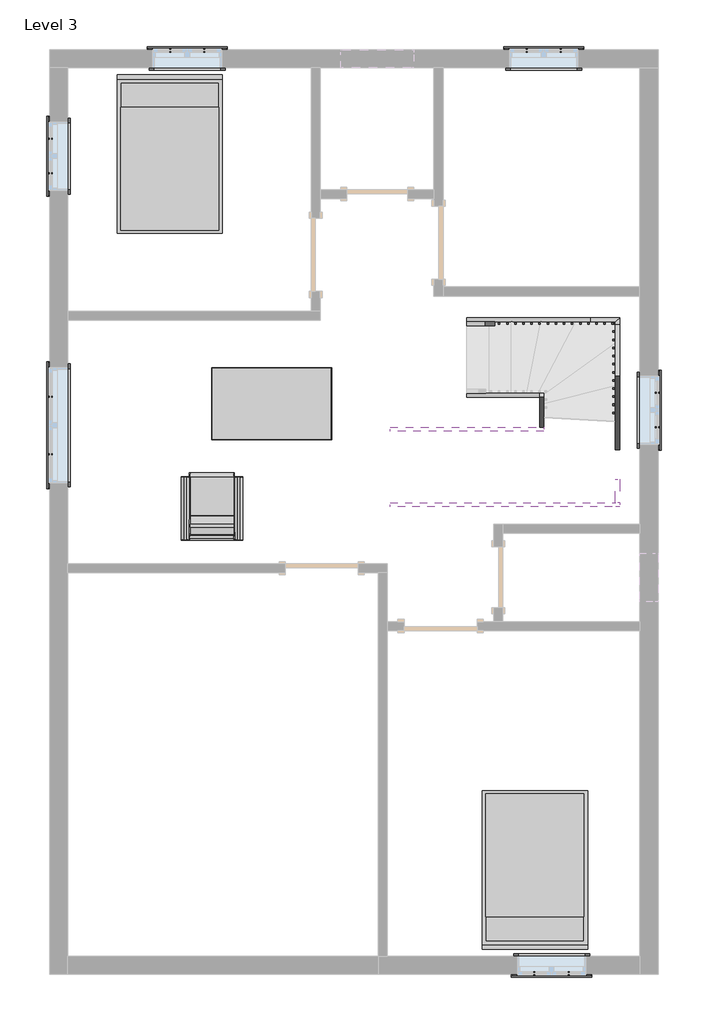
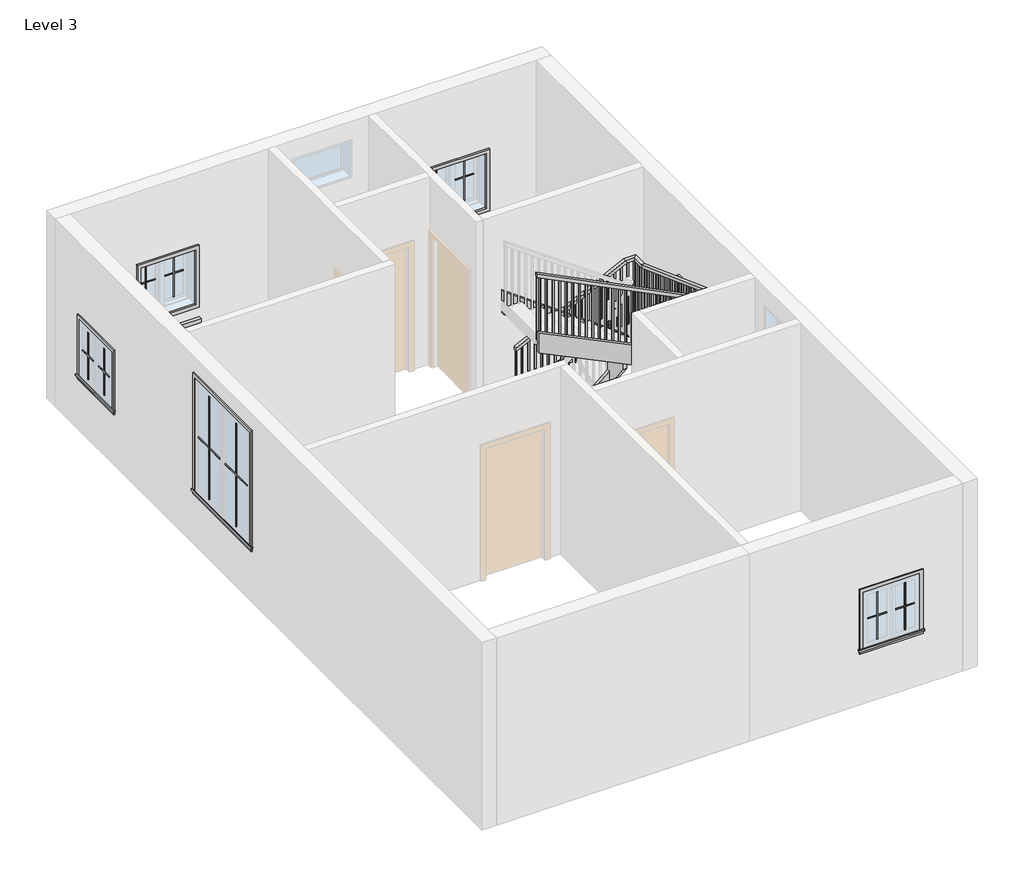
# One storey, part 2 of 2: 24 proxies, 9 members, 4 furniture elements, 1 railing.
"""IFC4 building model written with IfcOpenShell, lengths in millimetres."""

from ifc_helpers import new_model, si_unit, frame, origin, place, context, project, spatial, polyline, outline, extrude, faceted_brep, transform, mapped, element, save
from components import muntin_pattern_2x2_muntin_pattern_2x2_b3fe6957, muntin_pattern_2x2_muntin_pattern_2x2_3e0ecaf2, muntin_pattern_2x2_muntin_pattern_2x2_bff912c5, muntin_pattern_2x2_muntin_pattern_2x2_c2194282, trim_window_exterior_flat_with_sill_41619996, trim_window_exterior_flat_with_sill_e04b3088, trim_window_interior_flat_picture_frame_51c85655, trim_window_interior_flat_picture_frame_2a7685fe, furniture_f28dd14e, furniture_402a1f5e, bed_17739_bed_17739_15c61121, dining_table_14755_dining_table_14755_d89cb775

model = new_model("IFC4")

# Units and contexts
model_context = context("Model", 3, world=origin())
ifc_project = project(units=[si_unit("LENGTHUNIT", "METRE", prefix="MILLI")], contexts=[model_context])

# Site, building, storey
site = spatial("IfcSite", under=ifc_project)
building = spatial("IfcBuilding", under=site)
storey = spatial("IfcBuildingStorey", under=building, Name="Level 3", Elevation=3200.4)

# Proxies
placement = place(None, origin())
muntin_pattern_2x2_muntin_pattern_2x2_shape = muntin_pattern_2x2_muntin_pattern_2x2_b3fe6957(model_context)
element("IfcBuildingElementProxy", 1, Name="Muntin Pattern_2x2 : Muntin Pattern_2x2", ObjectType="Muntin Pattern_2x2 : Muntin Pattern_2x2", at=placement, inside=storey, context=model_context, shape_type="MappedRepresentation", body=[
    mapped(muntin_pattern_2x2_muntin_pattern_2x2_shape, transform((-3555.5290084, 6319.8685985, 4184.65), x_axis=(1.0, 0.0, 0.0), y_axis=(0.0, 1.0, 0.0), z_axis=(0.0, 0.0, 1.0))),
])
element("IfcBuildingElementProxy", 2, Name="Muntin Pattern_2x2 : Muntin Pattern_2x2", ObjectType="Muntin Pattern_2x2 : Muntin Pattern_2x2", at=placement, inside=storey, context=model_context, shape_type="MappedRepresentation", body=[
    mapped(muntin_pattern_2x2_muntin_pattern_2x2_shape, transform((1435.5709916, -5243.4814015, 4184.65), x_axis=(-1.0, 0.0, 0.0), y_axis=(0.0, -1.0, 0.0), z_axis=(0.0, 0.0, 1.0))),
])
element("IfcBuildingElementProxy", 3, Name="Muntin Pattern_2x2 : Muntin Pattern_2x2", ObjectType="Muntin Pattern_2x2 : Muntin Pattern_2x2", at=placement, inside=storey, context=model_context, shape_type="MappedRepresentation", body=[
    mapped(muntin_pattern_2x2_muntin_pattern_2x2_shape, transform((2545.2334916, 2028.8560985, 4184.65), x_axis=(0.0, -1.0, 0.0), y_axis=(1.0, 0.0, 0.0), z_axis=(0.0, 0.0, 1.0))),
])
element("IfcBuildingElementProxy", 4, Name="Muntin Pattern_2x2 : Muntin Pattern_2x2", ObjectType="Muntin Pattern_2x2 : Muntin Pattern_2x2", at=placement, inside=storey, context=model_context, shape_type="MappedRepresentation", body=[
    mapped(muntin_pattern_2x2_muntin_pattern_2x2_shape, transform((908.5209916, 6319.8685985, 4184.65), x_axis=(1.0, 0.0, 0.0), y_axis=(0.0, 1.0, 0.0), z_axis=(0.0, 0.0, 1.0))),
])
element("IfcBuildingElementProxy", 5, Name="Muntin Pattern_2x2 : Muntin Pattern_2x2", ObjectType="Muntin Pattern_2x2 : Muntin Pattern_2x2", at=placement, inside=storey, context=model_context, shape_type="MappedRepresentation", body=[
    mapped(muntin_pattern_2x2_muntin_pattern_2x2_shape, transform((-5055.7165084, 4781.5810985, 4184.65), x_axis=(0.0, 1.0, 0.0), y_axis=(-1.0, 0.0, 0.0), z_axis=(0.0, 0.0, 1.0))),
])
muntin_pattern_2x2_muntin_pattern_2x2_2_shape = muntin_pattern_2x2_muntin_pattern_2x2_3e0ecaf2(model_context)
element("IfcBuildingElementProxy", 6, Name="Muntin Pattern_2x2 : Muntin Pattern_2x2", ObjectType="Muntin Pattern_2x2 : Muntin Pattern_2x2", at=placement, inside=storey, context=model_context, shape_type="MappedRepresentation", body=[
    mapped(muntin_pattern_2x2_muntin_pattern_2x2_2_shape, transform((-3126.9040084, 6319.8685985, 4184.65), x_axis=(-1.0, 0.0, 0.0), y_axis=(0.0, -1.0, 0.0), z_axis=(0.0, 0.0, 1.0))),
])
element("IfcBuildingElementProxy", 7, Name="Muntin Pattern_2x2 : Muntin Pattern_2x2", ObjectType="Muntin Pattern_2x2 : Muntin Pattern_2x2", at=placement, inside=storey, context=model_context, shape_type="MappedRepresentation", body=[
    mapped(muntin_pattern_2x2_muntin_pattern_2x2_2_shape, transform((1006.9459916, -5243.4814015, 4184.65), x_axis=(1.0, 0.0, 0.0), y_axis=(0.0, 1.0, 0.0), z_axis=(0.0, 0.0, 1.0))),
])
element("IfcBuildingElementProxy", 8, Name="Muntin Pattern_2x2 : Muntin Pattern_2x2", ObjectType="Muntin Pattern_2x2 : Muntin Pattern_2x2", at=placement, inside=storey, context=model_context, shape_type="MappedRepresentation", body=[
    mapped(muntin_pattern_2x2_muntin_pattern_2x2_2_shape, transform((2545.2334916, 1600.2310985, 4184.65), x_axis=(0.0, 1.0, 0.0), y_axis=(-1.0, 0.0, 0.0), z_axis=(0.0, 0.0, 1.0))),
])
element("IfcBuildingElementProxy", 9, Name="Muntin Pattern_2x2 : Muntin Pattern_2x2", ObjectType="Muntin Pattern_2x2 : Muntin Pattern_2x2", at=placement, inside=storey, context=model_context, shape_type="MappedRepresentation", body=[
    mapped(muntin_pattern_2x2_muntin_pattern_2x2_2_shape, transform((1337.1459916, 6319.8685985, 4184.65), x_axis=(-1.0, 0.0, 0.0), y_axis=(0.0, -1.0, 0.0), z_axis=(0.0, 0.0, 1.0))),
])
element("IfcBuildingElementProxy", 10, Name="Muntin Pattern_2x2 : Muntin Pattern_2x2", ObjectType="Muntin Pattern_2x2 : Muntin Pattern_2x2", at=placement, inside=storey, context=model_context, shape_type="MappedRepresentation", body=[
    mapped(muntin_pattern_2x2_muntin_pattern_2x2_2_shape, transform((-5055.7165084, 5210.2060985, 4184.65), x_axis=(0.0, -1.0, 0.0), y_axis=(1.0, 0.0, 0.0), z_axis=(0.0, 0.0, 1.0))),
])
muntin_pattern_2x2_muntin_pattern_2x2_3_shape = muntin_pattern_2x2_muntin_pattern_2x2_bff912c5(model_context)
element("IfcBuildingElementProxy", 11, Name="Muntin Pattern_2x2 : Muntin Pattern_2x2", ObjectType="Muntin Pattern_2x2 : Muntin Pattern_2x2", at=placement, inside=storey, context=model_context, shape_type="MappedRepresentation", body=[
    mapped(muntin_pattern_2x2_muntin_pattern_2x2_3_shape, transform((-5055.7165084, 1263.6810985, 4184.65), x_axis=(0.0, 1.0, 0.0), y_axis=(-1.0, 0.0, 0.0), z_axis=(0.0, 0.0, 1.0))),
])
muntin_pattern_2x2_muntin_pattern_2x2_4_shape = muntin_pattern_2x2_muntin_pattern_2x2_c2194282(model_context)
element("IfcBuildingElementProxy", 12, Name="Muntin Pattern_2x2 : Muntin Pattern_2x2", ObjectType="Muntin Pattern_2x2 : Muntin Pattern_2x2", at=placement, inside=storey, context=model_context, shape_type="MappedRepresentation", body=[
    mapped(muntin_pattern_2x2_muntin_pattern_2x2_4_shape, transform((-5055.7165084, 1984.4060985, 4184.65), x_axis=(0.0, -1.0, 0.0), y_axis=(1.0, 0.0, 0.0), z_axis=(0.0, 0.0, 1.0))),
])
trim_window_exterior_flat_with_sill_shape = trim_window_exterior_flat_with_sill_41619996(model_context)
element("IfcBuildingElementProxy", 13, Name="Trim-Window-Exterior-Flat : with Sill", ObjectType="Trim-Window-Exterior-Flat : with Sill", at=placement, inside=storey, context=model_context, shape_type="MappedRepresentation", body=[
    mapped(trim_window_exterior_flat_with_sill_shape, transform((-3341.2165084, 6329.3935985, 5029.2), x_axis=(-1.0, 0.0, 0.0), y_axis=(0.0, 0.0, 1.0), z_axis=(0.0, 1.0, 0.0))),
])
element("IfcBuildingElementProxy", 14, Name="Trim-Window-Exterior-Flat : with Sill", ObjectType="Trim-Window-Exterior-Flat : with Sill", at=placement, inside=storey, context=model_context, shape_type="MappedRepresentation", body=[
    mapped(trim_window_exterior_flat_with_sill_shape, transform((1221.2584916, -5253.0064015, 5029.2), x_axis=(1.0, 0.0, 0.0), y_axis=(0.0, 0.0, 1.0), z_axis=(0.0, -1.0, 0.0))),
])
element("IfcBuildingElementProxy", 15, Name="Trim-Window-Exterior-Flat : with Sill", ObjectType="Trim-Window-Exterior-Flat : with Sill", at=placement, inside=storey, context=model_context, shape_type="MappedRepresentation", body=[
    mapped(trim_window_exterior_flat_with_sill_shape, transform((2554.7584916, 1814.5435985, 5029.2), x_axis=(0.0, 1.0, 0.0), y_axis=(0.0, 0.0, 1.0), z_axis=(1.0, 0.0, 0.0))),
])
element("IfcBuildingElementProxy", 16, Name="Trim-Window-Exterior-Flat : with Sill", ObjectType="Trim-Window-Exterior-Flat : with Sill", at=placement, inside=storey, context=model_context, shape_type="MappedRepresentation", body=[
    mapped(trim_window_exterior_flat_with_sill_shape, transform((1122.8334916, 6329.3935985, 5029.2), x_axis=(-1.0, 0.0, 0.0), y_axis=(0.0, 0.0, 1.0), z_axis=(0.0, 1.0, 0.0))),
])
element("IfcBuildingElementProxy", 17, Name="Trim-Window-Exterior-Flat : with Sill", ObjectType="Trim-Window-Exterior-Flat : with Sill", at=placement, inside=storey, context=model_context, shape_type="MappedRepresentation", body=[
    mapped(trim_window_exterior_flat_with_sill_shape, transform((-5065.2415084, 4995.8935985, 5029.2), x_axis=(0.0, -1.0, 0.0), y_axis=(0.0, 0.0, 1.0), z_axis=(-1.0, 0.0, 0.0))),
])
trim_window_exterior_flat_with_sill_2_shape = trim_window_exterior_flat_with_sill_e04b3088(model_context)
element("IfcBuildingElementProxy", 18, Name="Trim-Window-Exterior-Flat : with Sill", ObjectType="Trim-Window-Exterior-Flat : with Sill", at=placement, inside=storey, context=model_context, shape_type="MappedRepresentation", body=[
    mapped(trim_window_exterior_flat_with_sill_2_shape, transform((-5065.2415084, 1624.0435985, 5943.6), x_axis=(0.0, -1.0, 0.0), y_axis=(0.0, 0.0, 1.0), z_axis=(-1.0, 0.0, 0.0))),
])
trim_window_interior_flat_picture_frame_shape = trim_window_interior_flat_picture_frame_51c85655(model_context)
element("IfcBuildingElementProxy", 19, Name="Trim-Window-Interior-Flat : Picture Frame", ObjectType="Trim-Window-Interior-Flat : Picture Frame", at=placement, inside=storey, context=model_context, shape_type="MappedRepresentation", body=[
    mapped(trim_window_interior_flat_picture_frame_shape, transform((-3341.2165084, 6100.7935985, 5029.2), x_axis=(1.0, 0.0, 0.0), y_axis=(0.0, 0.0, 1.0), z_axis=(0.0, -1.0, 0.0))),
])
element("IfcBuildingElementProxy", 20, Name="Trim-Window-Interior-Flat : Picture Frame", ObjectType="Trim-Window-Interior-Flat : Picture Frame", at=placement, inside=storey, context=model_context, shape_type="MappedRepresentation", body=[
    mapped(trim_window_interior_flat_picture_frame_shape, transform((1221.2584916, -5024.4064015, 5029.2), x_axis=(-1.0, 0.0, 0.0), y_axis=(0.0, 0.0, 1.0), z_axis=(0.0, 1.0, 0.0))),
])
element("IfcBuildingElementProxy", 21, Name="Trim-Window-Interior-Flat : Picture Frame", ObjectType="Trim-Window-Interior-Flat : Picture Frame", at=placement, inside=storey, context=model_context, shape_type="MappedRepresentation", body=[
    mapped(trim_window_interior_flat_picture_frame_shape, transform((2326.1584916, 1814.5435985, 5029.2), x_axis=(0.0, -1.0, 0.0), y_axis=(0.0, 0.0, 1.0), z_axis=(-1.0, 0.0, 0.0))),
])
element("IfcBuildingElementProxy", 22, Name="Trim-Window-Interior-Flat : Picture Frame", ObjectType="Trim-Window-Interior-Flat : Picture Frame", at=placement, inside=storey, context=model_context, shape_type="MappedRepresentation", body=[
    mapped(trim_window_interior_flat_picture_frame_shape, transform((1122.8334916, 6100.7935985, 5029.2), x_axis=(1.0, 0.0, 0.0), y_axis=(0.0, 0.0, 1.0), z_axis=(0.0, -1.0, 0.0))),
])
element("IfcBuildingElementProxy", 23, Name="Trim-Window-Interior-Flat : Picture Frame", ObjectType="Trim-Window-Interior-Flat : Picture Frame", at=placement, inside=storey, context=model_context, shape_type="MappedRepresentation", body=[
    mapped(trim_window_interior_flat_picture_frame_shape, transform((-4836.6415084, 4995.8935985, 5029.2), x_axis=(0.0, 1.0, 0.0), y_axis=(0.0, 0.0, 1.0), z_axis=(1.0, 0.0, 0.0))),
])
trim_window_interior_flat_picture_frame_2_shape = trim_window_interior_flat_picture_frame_2a7685fe(model_context)
element("IfcBuildingElementProxy", 24, Name="Trim-Window-Interior-Flat : Picture Frame", ObjectType="Trim-Window-Interior-Flat : Picture Frame", at=placement, inside=storey, context=model_context, shape_type="MappedRepresentation", body=[
    mapped(trim_window_interior_flat_picture_frame_2_shape, transform((-4836.6415084, 1624.0435985, 5943.6), x_axis=(0.0, 1.0, 0.0), y_axis=(0.0, 0.0, 1.0), z_axis=(1.0, 0.0, 0.0))),
])

# Furniture
furniture_shape = furniture_f28dd14e(model_context)
furniture_2_shape = furniture_402a1f5e(model_context)
element("IfcFurniture", 25, at=placement, inside=storey, context=model_context, shape_type="MappedRepresentation", body=[
    mapped(furniture_shape, transform((-3032.3877006, 981.9349825, 3200.4), x_axis=(-1.0, 0.0, 0.0), y_axis=(0.0, -1.0, 0.0), z_axis=(0.0, 0.0, 1.0))),
    mapped(furniture_2_shape, transform((-3032.3877006, 981.9349825, 3200.4), x_axis=(-1.0, 0.0, 0.0), y_axis=(0.0, -1.0, 0.0), z_axis=(0.0, 0.0, 1.0))),
])
bed_17739_bed_17739_shape = bed_17739_bed_17739_15c61121(model_context)
element("IfcFurniture", 26, ObjectType="Bed_17739 : Bed_17739", at=placement, inside=storey, context=model_context, shape_type="MappedRepresentation", body=[
    mapped(bed_17739_bed_17739_shape, transform((-3560.2915084, 4995.8935985, 3200.4), x_axis=(1.0, 0.0, 0.0), y_axis=(0.0, 1.0, 0.0), z_axis=(0.0, 0.0, 1.0))),
])
element("IfcFurniture", 27, ObjectType="Bed_17739 : Bed_17739", at=placement, inside=storey, context=model_context, shape_type="MappedRepresentation", body=[
    mapped(bed_17739_bed_17739_shape, transform((1011.7084916, -3919.5064015, 3200.4), x_axis=(-1.0, 0.0, 0.0), y_axis=(0.0, -1.0, 0.0), z_axis=(0.0, 0.0, 1.0))),
])
dining_table_14755_dining_table_14755_shape = dining_table_14755_dining_table_14755_d89cb775(model_context)
element("IfcFurniture", 28, ObjectType="Dining_table_14755 : Dining_table_14755", at=placement, inside=storey, context=model_context, shape_type="MappedRepresentation", body=[
    mapped(dining_table_14755_dining_table_14755_shape, transform((-3032.3877006, 1444.8879061, 3200.4), x_axis=(1.0, 0.0, 0.0), y_axis=(0.0, 1.0, 0.0), z_axis=(0.0, 0.0, 1.0))),
])

# Members
element("IfcMember", 29, ObjectType="Stringer - 2\" Width", at=placement, inside=storey, context=model_context, shape_type="SweptSolid", body=[
    extrude(outline(polyline([(3439.8504763, 158.6923968), (3200.4, 158.6923968), (3200.4, 366.2169505), (3826.6639814, 1705.9967367), (4163.1193197, 1705.9967367), (3439.8504763, 158.6923968)])), frame((0.0, 2922.8476133, 0.0), z_axis=(0.0, 1.0, 0.0), x_axis=(0.0, 0.0, 1.0)), (0.0, 0.0, 1.0), 50.8),
])
element("IfcMember", 30, ObjectType="Stringer - 2\" Width", at=placement, inside=storey, context=model_context, shape_type="SweptSolid", body=[
    extrude(outline(polyline([(1705.9967367, 2922.8476133), (1705.9967367, 2973.6476133), (2072.9441983, 2973.6476133), (2022.1441983, 2922.8476133), (1705.9967367, 2922.8476133)])), frame((0.0, 0.0, 3826.6639814), z_axis=(0.0, 0.0, 1.0), x_axis=(1.0, 0.0, 0.0)), (0.0, 0.0, 1.0), 336.4553383),
])
element("IfcMember", 31, ObjectType="Stringer - 2\" Width", at=placement, inside=storey, context=model_context, shape_type="SweptSolid", body=[
    extrude(outline(polyline([(2022.1441983, 2922.8476133), (2072.9441983, 2973.6476133), (2072.9441983, 2883.4348143), (2022.1441983, 2883.4348143), (2022.1441983, 2922.8476133)])), frame((0.0, 0.0, 3826.6639814), z_axis=(0.0, 0.0, 1.0), x_axis=(1.0, 0.0, 0.0)), (0.0, 0.0, 1.0), 336.4553383),
])
element("IfcMember", 32, ObjectType="Stringer - 2\" Width", at=placement, inside=storey, context=model_context, shape_type="SweptSolid", body=[
    extrude(outline(polyline([(2883.4348143, 4163.1193197), (2883.4348143, 3826.6639814), (947.0260734, 4536.0990218), (947.0260734, 4872.5543601), (2883.4348143, 4163.1193197)])), frame((2022.1441983, 0.0, 0.0), z_axis=(1.0, 0.0, 0.0), x_axis=(0.0, 1.0, 0.0)), (0.0, 0.0, 1.0), 50.8),
])
element("IfcMember", 33, ObjectType="Stringer - 2\" Width", at=placement, inside=storey, context=model_context, shape_type="SweptSolid", body=[
    extrude(outline(polyline([(2022.1441983, 947.0260734), (2072.9441983, 947.0260734), (2072.9441983, 652.4935985), (2022.1441983, 652.4935985), (2022.1441983, 947.0260734)])), frame((0.0, 0.0, 4541.7754285), z_axis=(0.0, 0.0, 1.0), x_axis=(1.0, 0.0, 0.0)), (0.0, 0.0, 1.0), 324.6119022),
])
element("IfcMember", 34, ObjectType="Stringer - 2\" Width", at=placement, inside=storey, context=model_context, shape_type="SweptSolid", body=[
    extrude(outline(polyline([(3374.8551137, 158.6923968), (3200.4, 158.6923968), (3200.4, 426.0767146), (3734.5870321, 1072.5901835), (4129.9706215, 1072.5901835), (3374.8551137, 158.6923968)])), frame((0.0, 1973.2935985, 0.0), z_axis=(0.0, 1.0, 0.0), x_axis=(0.0, 0.0, 1.0)), (0.0, 0.0, 1.0), 50.8),
])
element("IfcMember", 35, ObjectType="Stringer - 2\" Width", at=placement, inside=storey, context=model_context, shape_type="SweptSolid", body=[
    extrude(outline(polyline([(2024.0935985, 4333.296008), (2024.0935985, 3830.5724164), (1602.0476133, 4384.1407029), (1602.0476133, 4886.8642945), (2024.0935985, 4333.296008)])), frame((1072.5901835, 0.0, 0.0), z_axis=(1.0, 0.0, 0.0), x_axis=(0.0, 1.0, 0.0)), (0.0, 0.0, 1.0), 50.8),
])
element("IfcMember", 36, ObjectType="Stringer - 2\" Width", at=placement, inside=storey, context=model_context, shape_type="SweptSolid", body=[
    extrude(outline(polyline([(4562.5113348, 1123.3901835), (4939.4379401, 1123.3901835), (6337.5009734, -798.3242294), (5960.5743681, -798.3242294), (4562.5113348, 1123.3901835)])), frame((0.0, 1551.2476133, 0.0), z_axis=(0.0, 1.0, 0.0), x_axis=(0.0, 0.0, 1.0)), (0.0, 0.0, 1.0), 50.8),
])
element("IfcMember", 37, ObjectType="Stringer - 2\" Width", at=placement, inside=storey, context=model_context, shape_type="SweptSolid", body=[
    extrude(outline(polyline([(4561.5873308, 2072.9441983), (4841.6397747, 2072.9441983), (6240.3971818, -798.3242294), (5915.7852796, -798.3242294), (4561.5873308, 1981.4757528), (4561.5873308, 2072.9441983)])), frame((0.0, 601.6935985, 0.0), z_axis=(0.0, 1.0, 0.0), x_axis=(0.0, 0.0, 1.0)), (0.0, 0.0, 1.0), 50.8),
])

# Railing
element("IfcRailing", 38, ObjectType="Handrail - Rectangular", at=placement, inside=storey, context=model_context, shape_type="SolidModel", body=[
    faceted_brep([(158.6923968, 2922.8476133, 4284.1333333), (158.6923968, 2922.8476133, 4227.4325724), (158.6923968, 2872.0476133, 4227.4325724), (158.6923968, 2872.0476133, 4284.1333333), (1841.0143863, 2922.8476133, 5118.2084972), (1852.9161672, 2922.8476133, 5067.4084972), (1852.9161672, 2872.0476133, 5067.4084972), (1841.0143863, 2872.0476133, 5118.2084972), (2022.1441983, 2922.8476133, 5118.2084972), (2022.1441983, 2922.8476133, 5067.4084972), (1971.3441983, 2872.0476133, 5067.4084972), (1971.3441983, 2872.0476133, 5118.2084972), (2022.1441983, 2686.7050655, 5118.2084972), (2022.1441983, 2677.692274, 5067.4084972), (1971.3441983, 2677.692274, 5067.4084972), (1971.3441983, 2686.7050655, 5118.2084972), (2022.1441983, 796.951655, 5810.5505936), (2022.1441983, 787.9388635, 5759.7505936), (1971.3441983, 787.9388635, 5759.7505936), (1971.3441983, 796.951655, 5810.5505936), (2022.1441983, 652.4935985, 5810.5505936), (2022.1441983, 652.4935985, 5759.7505936), (1971.3441983, 703.2935985, 5759.7505936), (1971.3441983, 703.2935985, 5810.5505936), (1909.402346, 652.4935985, 5810.5505936), (1897.4228813, 652.4935985, 5759.7505936), (1897.4228813, 703.2935985, 5759.7505936), (1909.402346, 703.2935985, 5810.5505936), (-798.3242294, 652.4935985, 7162.8), (-798.3242294, 703.2935985, 7162.8), (-798.3242294, 703.2935985, 7106.0174077), (-798.3242294, 652.4935985, 7106.0174077)], [[[0, 1, 2, 3]], [[1, 0, 4, 5]], [[2, 1, 5, 6]], [[3, 2, 6, 7]], [[0, 3, 7, 4]], [[5, 4, 8, 9]], [[6, 5, 9, 10]], [[7, 6, 10, 11]], [[4, 7, 11, 8]], [[9, 8, 12, 13]], [[10, 9, 13, 14]], [[11, 10, 14, 15]], [[8, 11, 15, 12]], [[13, 12, 16, 17]], [[14, 13, 17, 18]], [[15, 14, 18, 19]], [[12, 15, 19, 16]], [[17, 16, 20, 21]], [[18, 17, 21, 22]], [[19, 18, 22, 23]], [[16, 19, 23, 20]], [[21, 20, 24, 25]], [[22, 21, 25, 26]], [[23, 22, 26, 27]], [[20, 23, 27, 24]], [[28, 29, 30, 31]], [[25, 24, 28, 31]], [[26, 25, 31, 30]], [[27, 26, 30, 29]], [[24, 27, 29, 28]]]),
    extrude(outline(polyline([(7084.8709318, -755.9808017), (6079.0666667, -755.9808017), (6079.0666667, -736.9308017), (7075.3572862, -736.9308017), (7084.8709318, -755.9808017)])), frame((0.0, 668.3685985, 0.0), z_axis=(0.0, 1.0, 0.0), x_axis=(0.0, 0.0, 1.0)), (0.0, 0.0, 1.0), 19.05),
    extrude(outline(polyline([(7034.1314883, -654.3808017), (6079.0666667, -654.3808017), (6079.0666667, -635.3308017), (7024.6178426, -635.3308017), (7034.1314883, -654.3808017)])), frame((0.0, 668.3685985, 0.0), z_axis=(0.0, 1.0, 0.0), x_axis=(0.0, 0.0, 1.0)), (0.0, 0.0, 1.0), 19.05),
    extrude(outline(polyline([(6983.3920447, -552.7808017), (6079.0666667, -552.7808017), (6079.0666667, -533.7308017), (6973.8783991, -533.7308017), (6983.3920447, -552.7808017)])), frame((0.0, 668.3685985, 0.0), z_axis=(0.0, 1.0, 0.0), x_axis=(0.0, 0.0, 1.0)), (0.0, 0.0, 1.0), 19.05),
    extrude(outline(polyline([(6932.6526012, -451.1808017), (5909.7333333, -451.1808017), (5909.7333333, -432.1308017), (6923.1389555, -432.1308017), (6932.6526012, -451.1808017)])), frame((0.0, 668.3685985, 0.0), z_axis=(0.0, 1.0, 0.0), x_axis=(0.0, 0.0, 1.0)), (0.0, 0.0, 1.0), 19.05),
    extrude(outline(polyline([(6881.9131577, -349.5808017), (5909.7333333, -349.5808017), (5909.7333333, -330.5308017), (6872.399512, -330.5308017), (6881.9131577, -349.5808017)])), frame((0.0, 668.3685985, 0.0), z_axis=(0.0, 1.0, 0.0), x_axis=(0.0, 0.0, 1.0)), (0.0, 0.0, 1.0), 19.05),
    extrude(outline(polyline([(6831.1737141, -247.9808017), (5740.4, -247.9808017), (5740.4, -228.9308017), (6821.6600685, -228.9308017), (6831.1737141, -247.9808017)])), frame((0.0, 668.3685985, 0.0), z_axis=(0.0, 1.0, 0.0), x_axis=(0.0, 0.0, 1.0)), (0.0, 0.0, 1.0), 19.05),
    extrude(outline(polyline([(6780.4342706, -146.3808017), (5740.4, -146.3808017), (5740.4, -127.3308017), (6770.9206249, -127.3308017), (6780.4342706, -146.3808017)])), frame((0.0, 668.3685985, 0.0), z_axis=(0.0, 1.0, 0.0), x_axis=(0.0, 0.0, 1.0)), (0.0, 0.0, 1.0), 19.05),
    extrude(outline(polyline([(6729.694827, -44.7808017), (5740.4, -44.7808017), (5740.4, -25.7308017), (6720.1811814, -25.7308017), (6729.694827, -44.7808017)])), frame((0.0, 668.3685985, 0.0), z_axis=(0.0, 1.0, 0.0), x_axis=(0.0, 0.0, 1.0)), (0.0, 0.0, 1.0), 19.05),
    extrude(outline(polyline([(6678.9553835, 56.8191983), (5571.0666667, 56.8191983), (5571.0666667, 75.8691983), (6669.4417378, 75.8691983), (6678.9553835, 56.8191983)])), frame((0.0, 668.3685985, 0.0), z_axis=(0.0, 1.0, 0.0), x_axis=(0.0, 0.0, 1.0)), (0.0, 0.0, 1.0), 19.05),
    extrude(outline(polyline([(6628.21594, 158.4191983), (5571.0666667, 158.4191983), (5571.0666667, 177.4691983), (6618.7022943, 177.4691983), (6628.21594, 158.4191983)])), frame((0.0, 668.3685985, 0.0), z_axis=(0.0, 1.0, 0.0), x_axis=(0.0, 0.0, 1.0)), (0.0, 0.0, 1.0), 19.05),
    extrude(outline(polyline([(6577.4764964, 260.0191983), (5571.0666667, 260.0191983), (5571.0666667, 279.0691983), (6567.9628508, 279.0691983), (6577.4764964, 260.0191983)])), frame((0.0, 668.3685985, 0.0), z_axis=(0.0, 1.0, 0.0), x_axis=(0.0, 0.0, 1.0)), (0.0, 0.0, 1.0), 19.05),
    extrude(outline(polyline([(6526.7370529, 361.6191983), (5401.7333333, 361.6191983), (5401.7333333, 380.6691983), (6517.2234072, 380.6691983), (6526.7370529, 361.6191983)])), frame((0.0, 668.3685985, 0.0), z_axis=(0.0, 1.0, 0.0), x_axis=(0.0, 0.0, 1.0)), (0.0, 0.0, 1.0), 19.05),
    extrude(outline(polyline([(6475.9976093, 463.2191983), (5401.7333333, 463.2191983), (5401.7333333, 482.2691983), (6466.4839637, 482.2691983), (6475.9976093, 463.2191983)])), frame((0.0, 668.3685985, 0.0), z_axis=(0.0, 1.0, 0.0), x_axis=(0.0, 0.0, 1.0)), (0.0, 0.0, 1.0), 19.05),
    extrude(outline(polyline([(6425.2581658, 564.8191983), (5401.7333333, 564.8191983), (5401.7333333, 583.8691983), (6415.7445201, 583.8691983), (6425.2581658, 564.8191983)])), frame((0.0, 668.3685985, 0.0), z_axis=(0.0, 1.0, 0.0), x_axis=(0.0, 0.0, 1.0)), (0.0, 0.0, 1.0), 19.05),
    extrude(outline(polyline([(6374.5187223, 666.4191983), (5232.4, 666.4191983), (5232.4, 685.4691983), (6365.0050766, 685.4691983), (6374.5187223, 666.4191983)])), frame((0.0, 668.3685985, 0.0), z_axis=(0.0, 1.0, 0.0), x_axis=(0.0, 0.0, 1.0)), (0.0, 0.0, 1.0), 19.05),
    extrude(outline(polyline([(6323.7792787, 768.0191983), (5232.4, 768.0191983), (5232.4, 787.0691983), (6314.265633, 787.0691983), (6323.7792787, 768.0191983)])), frame((0.0, 668.3685985, 0.0), z_axis=(0.0, 1.0, 0.0), x_axis=(0.0, 0.0, 1.0)), (0.0, 0.0, 1.0), 19.05),
    extrude(outline(polyline([(6273.0398352, 869.6191983), (5232.4, 869.6191983), (5232.4, 888.6691983), (6263.5261895, 888.6691983), (6273.0398352, 869.6191983)])), frame((0.0, 668.3685985, 0.0), z_axis=(0.0, 1.0, 0.0), x_axis=(0.0, 0.0, 1.0)), (0.0, 0.0, 1.0), 19.05),
    extrude(outline(polyline([(6222.3003916, 971.2191983), (5232.4, 971.2191983), (5232.4, 990.2691983), (6212.786746, 990.2691983), (6222.3003916, 971.2191983)])), frame((0.0, 668.3685985, 0.0), z_axis=(0.0, 1.0, 0.0), x_axis=(0.0, 0.0, 1.0)), (0.0, 0.0, 1.0), 19.05),
    extrude(outline(polyline([(6171.5609481, 1072.8191983), (5063.0666667, 1072.8191983), (5063.0666667, 1091.8691983), (6162.0473024, 1091.8691983), (6171.5609481, 1072.8191983)])), frame((0.0, 668.3685985, 0.0), z_axis=(0.0, 1.0, 0.0), x_axis=(0.0, 0.0, 1.0)), (0.0, 0.0, 1.0), 19.05),
    extrude(outline(polyline([(6120.8215046, 1174.4191983), (5063.0666667, 1174.4191983), (5063.0666667, 1193.4691983), (6111.3078589, 1193.4691983), (6120.8215046, 1174.4191983)])), frame((0.0, 668.3685985, 0.0), z_axis=(0.0, 1.0, 0.0), x_axis=(0.0, 0.0, 1.0)), (0.0, 0.0, 1.0), 19.05),
    extrude(outline(polyline([(6070.082061, 1276.0191983), (5063.0666667, 1276.0191983), (5063.0666667, 1295.0691983), (6060.5684153, 1295.0691983), (6070.082061, 1276.0191983)])), frame((0.0, 668.3685985, 0.0), z_axis=(0.0, 1.0, 0.0), x_axis=(0.0, 0.0, 1.0)), (0.0, 0.0, 1.0), 19.05),
    extrude(outline(polyline([(6019.3426175, 1377.6191983), (4893.7333333, 1377.6191983), (4893.7333333, 1396.6691983), (6009.8289718, 1396.6691983), (6019.3426175, 1377.6191983)])), frame((0.0, 668.3685985, 0.0), z_axis=(0.0, 1.0, 0.0), x_axis=(0.0, 0.0, 1.0)), (0.0, 0.0, 1.0), 19.05),
    extrude(outline(polyline([(5968.6031739, 1479.2191983), (4893.7333333, 1479.2191983), (4893.7333333, 1498.2691983), (5959.0895283, 1498.2691983), (5968.6031739, 1479.2191983)])), frame((0.0, 668.3685985, 0.0), z_axis=(0.0, 1.0, 0.0), x_axis=(0.0, 0.0, 1.0)), (0.0, 0.0, 1.0), 19.05),
    extrude(outline(polyline([(5917.8637304, 1580.8191983), (4893.7333333, 1580.8191983), (4893.7333333, 1599.8691983), (5908.3500847, 1599.8691983), (5917.8637304, 1580.8191983)])), frame((0.0, 668.3685985, 0.0), z_axis=(0.0, 1.0, 0.0), x_axis=(0.0, 0.0, 1.0)), (0.0, 0.0, 1.0), 19.05),
    extrude(outline(polyline([(5867.1242869, 1682.4191983), (4893.7333333, 1682.4191983), (4893.7333333, 1701.4691983), (5857.6106412, 1701.4691983), (5867.1242869, 1682.4191983)])), frame((0.0, 668.3685985, 0.0), z_axis=(0.0, 1.0, 0.0), x_axis=(0.0, 0.0, 1.0)), (0.0, 0.0, 1.0), 19.05),
    extrude(outline(polyline([(5816.3848433, 1784.0191983), (4893.7333333, 1784.0191983), (4893.7333333, 1803.0691983), (5806.8711976, 1803.0691983), (5816.3848433, 1784.0191983)])), frame((0.0, 668.3685985, 0.0), z_axis=(0.0, 1.0, 0.0), x_axis=(0.0, 0.0, 1.0)), (0.0, 0.0, 1.0), 19.05),
    extrude(outline(polyline([(5765.6453998, 1885.6191983), (4724.4, 1885.6191983), (4724.4, 1904.6691983), (5756.1317541, 1904.6691983), (5765.6453998, 1885.6191983)])), frame((0.0, 668.3685985, 0.0), z_axis=(0.0, 1.0, 0.0), x_axis=(0.0, 0.0, 1.0)), (0.0, 0.0, 1.0), 19.05),
    extrude(outline(polyline([(2006.2691983, 773.3726133), (2006.2691983, 754.3226133), (1987.2191983, 754.3226133), (1987.2191983, 773.3726133), (2006.2691983, 773.3726133)])), frame((0.0, 0.0, 4724.4), z_axis=(0.0, 0.0, 1.0), x_axis=(1.0, 0.0, 0.0)), (0.0, 0.0, 1.0), 1035.3505936),
    extrude(outline(polyline([(874.9726133, 5727.8643546), (874.9726133, 4724.4), (855.9226133, 4724.4), (855.9226133, 5734.843634), (874.9726133, 5727.8643546)])), frame((1987.2191983, 0.0, 0.0), z_axis=(1.0, 0.0, 0.0), x_axis=(0.0, 1.0, 0.0)), (0.0, 0.0, 1.0), 19.05),
    extrude(outline(polyline([(976.5726133, 5690.6415315), (976.5726133, 4724.4), (957.5226133, 4724.4), (957.5226133, 5697.6208108), (976.5726133, 5690.6415315)])), frame((1987.2191983, 0.0, 0.0), z_axis=(1.0, 0.0, 0.0), x_axis=(0.0, 1.0, 0.0)), (0.0, 0.0, 1.0), 19.05),
    extrude(outline(polyline([(1078.1726133, 5653.4187083), (1078.1726133, 4724.4), (1059.1226133, 4724.4), (1059.1226133, 5660.3979877), (1078.1726133, 5653.4187083)])), frame((1987.2191983, 0.0, 0.0), z_axis=(1.0, 0.0, 0.0), x_axis=(0.0, 1.0, 0.0)), (0.0, 0.0, 1.0), 19.05),
    extrude(outline(polyline([(1179.7726133, 5616.1958852), (1179.7726133, 4724.4), (1160.7226133, 4724.4), (1160.7226133, 5623.1751645), (1179.7726133, 5616.1958852)])), frame((1987.2191983, 0.0, 0.0), z_axis=(1.0, 0.0, 0.0), x_axis=(0.0, 1.0, 0.0)), (0.0, 0.0, 1.0), 19.05),
    extrude(outline(polyline([(1281.3726133, 5578.973062), (1281.3726133, 4724.4), (1262.3226133, 4724.4), (1262.3226133, 5585.9523414), (1281.3726133, 5578.973062)])), frame((1987.2191983, 0.0, 0.0), z_axis=(1.0, 0.0, 0.0), x_axis=(0.0, 1.0, 0.0)), (0.0, 0.0, 1.0), 19.05),
    extrude(outline(polyline([(1382.9726133, 5541.7502389), (1382.9726133, 4555.0666667), (1363.9226133, 4555.0666667), (1363.9226133, 5548.7295182), (1382.9726133, 5541.7502389)])), frame((1987.2191983, 0.0, 0.0), z_axis=(1.0, 0.0, 0.0), x_axis=(0.0, 1.0, 0.0)), (0.0, 0.0, 1.0), 19.05),
    extrude(outline(polyline([(1484.5726133, 5504.5274157), (1484.5726133, 4555.0666667), (1465.5226133, 4555.0666667), (1465.5226133, 5511.5066951), (1484.5726133, 5504.5274157)])), frame((1987.2191983, 0.0, 0.0), z_axis=(1.0, 0.0, 0.0), x_axis=(0.0, 1.0, 0.0)), (0.0, 0.0, 1.0), 19.05),
    extrude(outline(polyline([(1586.1726133, 5467.3045926), (1586.1726133, 4555.0666667), (1567.1226133, 4555.0666667), (1567.1226133, 5474.2838719), (1586.1726133, 5467.3045926)])), frame((1987.2191983, 0.0, 0.0), z_axis=(1.0, 0.0, 0.0), x_axis=(0.0, 1.0, 0.0)), (0.0, 0.0, 1.0), 19.05),
    extrude(outline(polyline([(1687.7726133, 5430.0817694), (1687.7726133, 4555.0666667), (1668.7226133, 4555.0666667), (1668.7226133, 5437.0610488), (1687.7726133, 5430.0817694)])), frame((1987.2191983, 0.0, 0.0), z_axis=(1.0, 0.0, 0.0), x_axis=(0.0, 1.0, 0.0)), (0.0, 0.0, 1.0), 19.05),
    extrude(outline(polyline([(1789.3726133, 5392.8589463), (1789.3726133, 4385.7333333), (1770.3226133, 4385.7333333), (1770.3226133, 5399.8382256), (1789.3726133, 5392.8589463)])), frame((1987.2191983, 0.0, 0.0), z_axis=(1.0, 0.0, 0.0), x_axis=(0.0, 1.0, 0.0)), (0.0, 0.0, 1.0), 19.05),
    extrude(outline(polyline([(1890.9726133, 5355.6361231), (1890.9726133, 4385.7333333), (1871.9226133, 4385.7333333), (1871.9226133, 5362.6154025), (1890.9726133, 5355.6361231)])), frame((1987.2191983, 0.0, 0.0), z_axis=(1.0, 0.0, 0.0), x_axis=(0.0, 1.0, 0.0)), (0.0, 0.0, 1.0), 19.05),
    extrude(outline(polyline([(1992.5726133, 5318.4133), (1992.5726133, 4385.7333333), (1973.5226133, 4385.7333333), (1973.5226133, 5325.3925793), (1992.5726133, 5318.4133)])), frame((1987.2191983, 0.0, 0.0), z_axis=(1.0, 0.0, 0.0), x_axis=(0.0, 1.0, 0.0)), (0.0, 0.0, 1.0), 19.05),
    extrude(outline(polyline([(2094.1726133, 5281.1904769), (2094.1726133, 4385.7333333), (2075.1226133, 4385.7333333), (2075.1226133, 5288.1697562), (2094.1726133, 5281.1904769)])), frame((1987.2191983, 0.0, 0.0), z_axis=(1.0, 0.0, 0.0), x_axis=(0.0, 1.0, 0.0)), (0.0, 0.0, 1.0), 19.05),
    extrude(outline(polyline([(2195.7726133, 5243.9676537), (2195.7726133, 4216.4), (2176.7226133, 4216.4), (2176.7226133, 5250.946933), (2195.7726133, 5243.9676537)])), frame((1987.2191983, 0.0, 0.0), z_axis=(1.0, 0.0, 0.0), x_axis=(0.0, 1.0, 0.0)), (0.0, 0.0, 1.0), 19.05),
    extrude(outline(polyline([(2297.3726133, 5206.7448306), (2297.3726133, 4216.4), (2278.3226133, 4216.4), (2278.3226133, 5213.7241099), (2297.3726133, 5206.7448306)])), frame((1987.2191983, 0.0, 0.0), z_axis=(1.0, 0.0, 0.0), x_axis=(0.0, 1.0, 0.0)), (0.0, 0.0, 1.0), 19.05),
    extrude(outline(polyline([(2398.9726133, 5169.5220074), (2398.9726133, 4216.4), (2379.9226133, 4216.4), (2379.9226133, 5176.5012867), (2398.9726133, 5169.5220074)])), frame((1987.2191983, 0.0, 0.0), z_axis=(1.0, 0.0, 0.0), x_axis=(0.0, 1.0, 0.0)), (0.0, 0.0, 1.0), 19.05),
    extrude(outline(polyline([(2500.5726133, 5132.2991843), (2500.5726133, 4216.4), (2481.5226133, 4216.4), (2481.5226133, 5139.2784636), (2500.5726133, 5132.2991843)])), frame((1987.2191983, 0.0, 0.0), z_axis=(1.0, 0.0, 0.0), x_axis=(0.0, 1.0, 0.0)), (0.0, 0.0, 1.0), 19.05),
    extrude(outline(polyline([(2602.1726133, 5095.0763611), (2602.1726133, 4216.4), (2583.1226133, 4216.4), (2583.1226133, 5102.0556405), (2602.1726133, 5095.0763611)])), frame((1987.2191983, 0.0, 0.0), z_axis=(1.0, 0.0, 0.0), x_axis=(0.0, 1.0, 0.0)), (0.0, 0.0, 1.0), 19.05),
    extrude(outline(polyline([(2006.2691983, 2703.7726133), (2006.2691983, 2684.7226133), (1987.2191983, 2684.7226133), (1987.2191983, 2703.7726133), (2006.2691983, 2703.7726133)])), frame((0.0, 0.0, 4047.0666667), z_axis=(0.0, 0.0, 1.0), x_axis=(1.0, 0.0, 0.0)), (0.0, 0.0, 1.0), 1020.3418305),
    extrude(outline(polyline([(2006.2691983, 2805.3726133), (2006.2691983, 2786.3226133), (1987.2191983, 2786.3226133), (1987.2191983, 2805.3726133), (2006.2691983, 2805.3726133)])), frame((0.0, 0.0, 4047.0666667), z_axis=(0.0, 0.0, 1.0), x_axis=(1.0, 0.0, 0.0)), (0.0, 0.0, 1.0), 1020.3418305),
    extrude(outline(polyline([(1977.9673968, 2906.9726133), (1997.0173968, 2906.9726133), (1997.0173968, 2887.9226133), (1977.9673968, 2887.9226133), (1977.9673968, 2906.9726133)])), frame((0.0, 0.0, 4047.0666667), z_axis=(0.0, 0.0, 1.0), x_axis=(1.0, 0.0, 0.0)), (0.0, 0.0, 1.0), 1020.3418305),
    extrude(outline(polyline([(1876.3673968, 2906.9726133), (1895.4173968, 2906.9726133), (1895.4173968, 2887.9226133), (1876.3673968, 2887.9226133), (1876.3673968, 2906.9726133)])), frame((0.0, 0.0, 4047.0666667), z_axis=(0.0, 0.0, 1.0), x_axis=(1.0, 0.0, 0.0)), (0.0, 0.0, 1.0), 1020.3418305),
    extrude(outline(polyline([(5028.6632695, 1774.7673968), (4047.0666667, 1774.7673968), (4047.0666667, 1793.8173968), (5038.1080321, 1793.8173968), (5028.6632695, 1774.7673968)])), frame((0.0, 2887.9226133, 0.0), z_axis=(0.0, 1.0, 0.0), x_axis=(0.0, 0.0, 1.0)), (0.0, 0.0, 1.0), 19.05),
    extrude(outline(polyline([(4978.2912021, 1673.1673968), (4047.0666667, 1673.1673968), (4047.0666667, 1692.2173968), (4987.7359647, 1692.2173968), (4978.2912021, 1673.1673968)])), frame((0.0, 2887.9226133, 0.0), z_axis=(0.0, 1.0, 0.0), x_axis=(0.0, 0.0, 1.0)), (0.0, 0.0, 1.0), 19.05),
    extrude(outline(polyline([(4927.9191347, 1571.5673968), (4047.0666667, 1571.5673968), (4047.0666667, 1590.6173968), (4937.3638973, 1590.6173968), (4927.9191347, 1571.5673968)])), frame((0.0, 2887.9226133, 0.0), z_axis=(0.0, 1.0, 0.0), x_axis=(0.0, 0.0, 1.0)), (0.0, 0.0, 1.0), 19.05),
    extrude(outline(polyline([(4877.5470673, 1469.9673968), (3877.7333333, 1469.9673968), (3877.7333333, 1489.0173968), (4886.9918299, 1489.0173968), (4877.5470673, 1469.9673968)])), frame((0.0, 2887.9226133, 0.0), z_axis=(0.0, 1.0, 0.0), x_axis=(0.0, 0.0, 1.0)), (0.0, 0.0, 1.0), 19.05),
    extrude(outline(polyline([(4827.1749999, 1368.3673968), (3877.7333333, 1368.3673968), (3877.7333333, 1387.4173968), (4836.6197625, 1387.4173968), (4827.1749999, 1368.3673968)])), frame((0.0, 2887.9226133, 0.0), z_axis=(0.0, 1.0, 0.0), x_axis=(0.0, 0.0, 1.0)), (0.0, 0.0, 1.0), 19.05),
    extrude(outline(polyline([(4776.8029325, 1266.7673968), (3877.7333333, 1266.7673968), (3877.7333333, 1285.8173968), (4786.2476951, 1285.8173968), (4776.8029325, 1266.7673968)])), frame((0.0, 2887.9226133, 0.0), z_axis=(0.0, 1.0, 0.0), x_axis=(0.0, 0.0, 1.0)), (0.0, 0.0, 1.0), 19.05),
    extrude(outline(polyline([(4726.4308651, 1165.1673968), (3877.7333333, 1165.1673968), (3877.7333333, 1184.2173968), (4735.8756277, 1184.2173968), (4726.4308651, 1165.1673968)])), frame((0.0, 2887.9226133, 0.0), z_axis=(0.0, 1.0, 0.0), x_axis=(0.0, 0.0, 1.0)), (0.0, 0.0, 1.0), 19.05),
    extrude(outline(polyline([(4676.0587977, 1063.5673968), (3708.4, 1063.5673968), (3708.4, 1082.6173968), (4685.5035603, 1082.6173968), (4676.0587977, 1063.5673968)])), frame((0.0, 2887.9226133, 0.0), z_axis=(0.0, 1.0, 0.0), x_axis=(0.0, 0.0, 1.0)), (0.0, 0.0, 1.0), 19.05),
    extrude(outline(polyline([(4625.6867303, 961.9673968), (3708.4, 961.9673968), (3708.4, 981.0173968), (4635.1314929, 981.0173968), (4625.6867303, 961.9673968)])), frame((0.0, 2887.9226133, 0.0), z_axis=(0.0, 1.0, 0.0), x_axis=(0.0, 0.0, 1.0)), (0.0, 0.0, 1.0), 19.05),
    extrude(outline(polyline([(4575.3146629, 860.3673968), (3708.4, 860.3673968), (3708.4, 879.4173968), (4584.7594255, 879.4173968), (4575.3146629, 860.3673968)])), frame((0.0, 2887.9226133, 0.0), z_axis=(0.0, 1.0, 0.0), x_axis=(0.0, 0.0, 1.0)), (0.0, 0.0, 1.0), 19.05),
    extrude(outline(polyline([(4524.9425955, 758.7673968), (3708.4, 758.7673968), (3708.4, 777.8173968), (4534.3873581, 777.8173968), (4524.9425955, 758.7673968)])), frame((0.0, 2887.9226133, 0.0), z_axis=(0.0, 1.0, 0.0), x_axis=(0.0, 0.0, 1.0)), (0.0, 0.0, 1.0), 19.05),
    extrude(outline(polyline([(4474.5705281, 657.1673968), (3539.0666667, 657.1673968), (3539.0666667, 676.2173968), (4484.0152907, 676.2173968), (4474.5705281, 657.1673968)])), frame((0.0, 2887.9226133, 0.0), z_axis=(0.0, 1.0, 0.0), x_axis=(0.0, 0.0, 1.0)), (0.0, 0.0, 1.0), 19.05),
    extrude(outline(polyline([(4424.1984607, 555.5673968), (3539.0666667, 555.5673968), (3539.0666667, 574.6173968), (4433.6432233, 574.6173968), (4424.1984607, 555.5673968)])), frame((0.0, 2887.9226133, 0.0), z_axis=(0.0, 1.0, 0.0), x_axis=(0.0, 0.0, 1.0)), (0.0, 0.0, 1.0), 19.05),
    extrude(outline(polyline([(4373.8263933, 453.9673968), (3539.0666667, 453.9673968), (3539.0666667, 473.0173968), (4383.2711559, 473.0173968), (4373.8263933, 453.9673968)])), frame((0.0, 2887.9226133, 0.0), z_axis=(0.0, 1.0, 0.0), x_axis=(0.0, 0.0, 1.0)), (0.0, 0.0, 1.0), 19.05),
    extrude(outline(polyline([(4323.4543259, 352.3673968), (3369.7333333, 352.3673968), (3369.7333333, 371.4173968), (4332.8990885, 371.4173968), (4323.4543259, 352.3673968)])), frame((0.0, 2887.9226133, 0.0), z_axis=(0.0, 1.0, 0.0), x_axis=(0.0, 0.0, 1.0)), (0.0, 0.0, 1.0), 19.05),
    extrude(outline(polyline([(4273.0822585, 250.7673968), (3369.7333333, 250.7673968), (3369.7333333, 269.8173968), (4282.5270211, 269.8173968), (4273.0822585, 250.7673968)])), frame((0.0, 2887.9226133, 0.0), z_axis=(0.0, 1.0, 0.0), x_axis=(0.0, 0.0, 1.0)), (0.0, 0.0, 1.0), 19.05),
    extrude(outline(polyline([(2006.2691983, 687.4185985), (2006.2691983, 668.3685985), (1987.2191983, 668.3685985), (1987.2191983, 687.4185985), (2006.2691983, 687.4185985)])), frame((0.0, 0.0, 4724.4), z_axis=(0.0, 0.0, 1.0), x_axis=(1.0, 0.0, 0.0)), (0.0, 0.0, 1.0), 1035.3505936),
    extrude(outline(polyline([(1987.2191983, 2906.9726133), (2006.2691983, 2906.9726133), (2006.2691983, 2887.9226133), (1987.2191983, 2887.9226133), (1987.2191983, 2906.9726133)])), frame((0.0, 0.0, 4047.0666667), z_axis=(0.0, 0.0, 1.0), x_axis=(1.0, 0.0, 0.0)), (0.0, 0.0, 1.0), 1020.3418305),
    extrude(outline(polyline([(7106.0174077, -798.3242294), (6079.0666667, -798.3242294), (6079.0666667, -779.2742294), (7096.5037621, -779.2742294), (7106.0174077, -798.3242294)])), frame((0.0, 668.3685985, 0.0), z_axis=(0.0, 1.0, 0.0), x_axis=(0.0, 0.0, 1.0)), (0.0, 0.0, 1.0), 19.05),
    extrude(outline(polyline([(4227.4325724, 158.6923968), (3369.7333333, 158.6923968), (3369.7333333, 177.7423968), (4236.877335, 177.7423968), (4227.4325724, 158.6923968)])), frame((0.0, 2887.9226133, 0.0), z_axis=(0.0, 1.0, 0.0), x_axis=(0.0, 0.0, 1.0)), (0.0, 0.0, 1.0), 19.05),
])

save(model, "model.ifc")

# Revit data of these elements
# Type "Muntin Pattern_2x2 : Muntin Pattern_2x2"
#   Width [instance default] = 4' - 0"
#   Thickness = 0' - 0 1/2"
#   Height [instance default] = 4' - 0"
#   Distance = 0' - 0 3/4"
#   Interior Material [instance default] = none
#   Exterior Material [instance default] = none
#   Default Elevation = 0
# Type "Trim-Window-Exterior-Flat : with Sill"
#   Trim Width = 0' - 2 1/4"
#   Trim Thickness_Picture Frame = 0' - 1 1/4"
#   Trim Thickness_with Sill = 0' - 0 3/4"
#   Sill Thickness = 0' - 1 1/4"
#   Opening Width [instance default] = 2' - 0"
#   Opening Height [instance default] = 3' - 0"
#   Default Elevation = 4' - 0"
#   Sill = yes
#   Picture Frame = no
#   Trim Material [instance default] = none
# Type "Trim-Window-Interior-Flat : Picture Frame"
#   Trim Thickness_Picture Frame = 0' - 1 1/4"
#   Trim Width = 0' - 2 1/4"
#   Trim Thickness_with Sill = 0' - 0 3/4"
#   Sill Thickness = 0' - 1 1/4"
#   Opening Width [instance default] = 2' - 0"
#   Opening Height [instance default] = 3' - 0"
#   Default Elevation = 4' - 0"
#   Sill = no
#   Picture Frame = yes
#   Trim Material [instance default] = none
# Type
#   Width [instance] = 2' - 6.31496"
#   Default Elevation = 0
# Type "Bed_17739 : Bed_17739"
#   Default Elevation = 0
# Type "Dining_table_14755 : Dining_table_14755"
#   Lengte [instance default] = 4' - 11.05512"
#   Breedte [instance default] = 2' - 11.43307"
#   Tafelblad = none
#   Poten = none
#   Default Elevation = 0
# Type "Handrail - Rectangular"
#   Assembly Code = "C2010400"
#   built-in parameter 1008612 = 0.0416667 (stored number, unit not read)
#   built-in parameter 1008611 = 0.0416667 (stored number, unit not read)
#   built-in parameter 1008609 = 0.333333 (stored number, unit not read)
#   built-in parameter 1008604 = 0.166667 (stored number, unit not read)
#   built-in parameter 1008603 = 0.166667 (stored number, unit not read)
#   Railing Height = 3' - 0"
#   built-in parameter 1008630 = 2
#   built-in parameter 1008610 = 2
#   built-in parameter 1008618 = Baluster - Square : 3/4"
# Elements 1, 2, 3, 4, 5, 6, 7, 8, 9, 10 (IfcBuildingElementProxy, "Muntin Pattern_2x2 : Muntin Pattern_2x2")
#   Width = 0' - 11 5/8"
#   Height = 2' - 6 1/2"
#   Interior Material = Wood - Stained
#   Exterior Material = Clad - White
#   Phase Created = New Construction
#   Materials on its faces: "Clad - White", "Wood - Stained"
# Elements 11, 12 (IfcBuildingElementProxy, "Muntin Pattern_2x2 : Muntin Pattern_2x2")
#   Width = 1' - 11 1/8"
#   Height = 5' - 6 1/2"
#   Interior Material = Wood - Stained
#   Exterior Material = Clad - White
#   Phase Created = New Construction
#   Materials on its faces: "Clad - White", "Wood - Stained"
# Elements 13, 14, 15, 16, 17 (IfcBuildingElementProxy, "Trim-Window-Exterior-Flat : with Sill")
#   Opening Width = 2' - 10"
#   Opening Height = 3' - 0"
#   Trim Material = Clad - White
#   Phase Created = New Construction
#   Materials on its faces: "Clad - White"
# Element 18 (IfcBuildingElementProxy, "Trim-Window-Exterior-Flat : with Sill")
#   Opening Width = 4' - 9"
#   Opening Height = 6' - 0"
#   Trim Material = Clad - White
#   Phase Created = New Construction
#   Materials on its faces: "Clad - White"
# Elements 19, 20, 21, 22, 23 (IfcBuildingElementProxy, "Trim-Window-Interior-Flat : Picture Frame")
#   Opening Width = 2' - 10"
#   Opening Height = 3' - 0"
#   Trim Material = Wood - Stained
#   Phase Created = New Construction
#   Materials on its faces: "Wood - Stained"
# Element 24 (IfcBuildingElementProxy, "Trim-Window-Interior-Flat : Picture Frame")
#   Opening Width = 4' - 9"
#   Opening Height = 6' - 0"
#   Trim Material = Wood - Stained
#   Phase Created = New Construction
#   Materials on its faces: "Wood - Stained"
# Element 25 (IfcFurniture)
#   Width = 2' - 6.31496"
#   Phase Created = New Construction
# Elements 26, 27 (IfcFurniture, "Bed_17739 : Bed_17739")
#   Phase Created = New Construction
#   Materials on its faces: "legs", "sheets", "bed frame", "Blanket"
# Element 28 (IfcFurniture, "Dining_table_14755 : Dining_table_14755")
#   Lengte = 4' - 11.05512"
#   Breedte = 2' - 11.43307"
#   Phase Created = New Construction
# Elements 29, 30, 31, 32, 33, 34, 35, 36, 37 (IfcMember, "Stringer - 2\" Width")
#   Phase Created = New Construction
# Element 38 (IfcRailing, "Handrail - Rectangular")
#   Phase Created = New Construction
# Materials
#   "Clad - White": class "Wood", colour RGB 242 242 238, transparency 0, Cost = 0
#   "Wood - Stained": class "Wood", colour RGB 224 178 126, transparency 0, Cost = 0
#   "legs": colour RGB 90 73 37, transparency 0, Cost = 0
#   "sheets": colour RGB 200 195 176, transparency 0, Cost = 0
#   "bed frame": colour RGB 90 73 37, transparency 0, Cost = 0
#   "Blanket": class "System", colour RGB 59 0 1, transparency 0, Cost = 0
